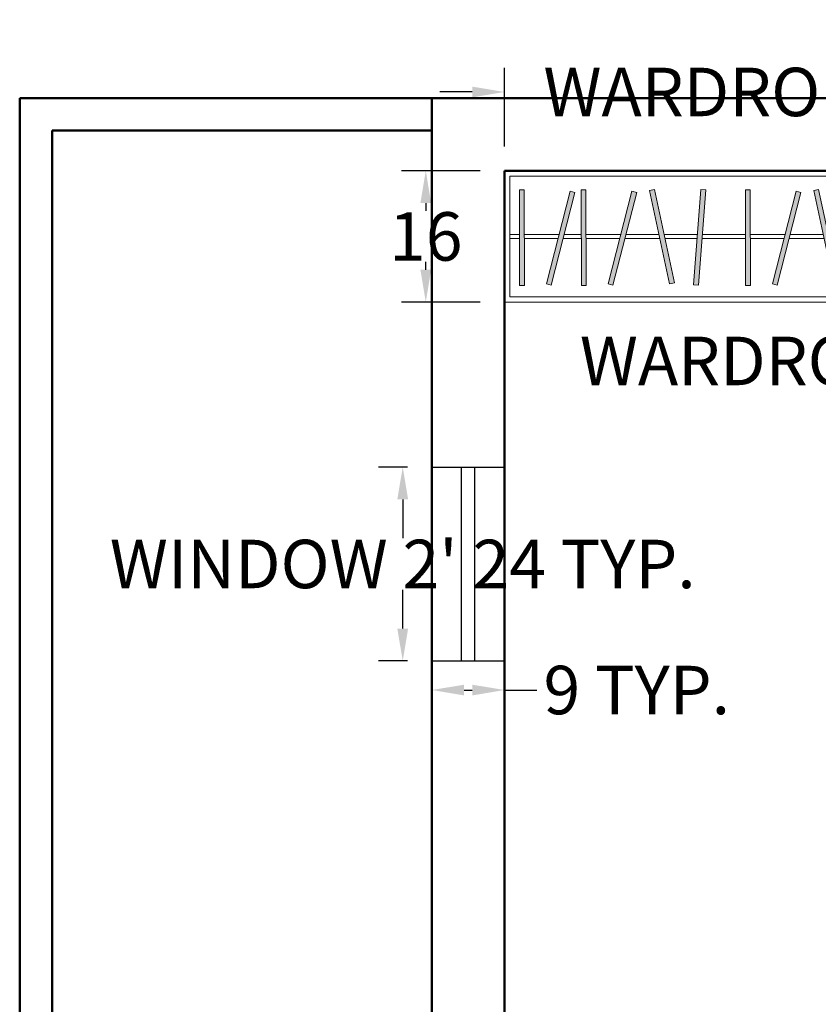
# Model space of a CAD drawing. Units: inches. Extents: x -466983 to 1020, y 324 to 318697.
# Tile 45 of 97: x 392 to 491, y 973 to 1095. Entities that reach past the tile are written whole.
import ezdxf

# ---------------------------------------------------------------- set-up
doc = ezdxf.new("R2010")
doc.units = ezdxf.units.IN
doc.header["$MEASUREMENT"] = 0
for name, color, linetype, lineweight in [('A-ANNO-DIMS', 2, 'Continuous', 18), ('A-ANNO-TEXT', 7, 'Continuous', 18), ('A-FLOR-PATT', 252, 'Continuous', 13), ('A-FURN', 8, 'Continuous', 18), ('A-GLAZ', 4, 'Continuous', 25), ('A-WALL', 7, 'Continuous', 50)]:
    doc.layers.add(name, color=color, linetype=linetype, lineweight=lineweight)
doc.styles.get("Standard").update_dxf_attribs({"font": 'arial.ttf'})
doc.dimstyles.get("Standard").update_dxf_attribs({"dimtxt": 6, "dimasz": 4, "dimexe": 3, "dimexo": 3, "dimgap": 0.09, "dimtad": 0, "dimtih": 1, "dimtoh": 1, "dimdec": 1, "dimzin": 0, "dimdsep": 46, "dimlunit": 3, "dimtxsty": 'Standard', "dimcen": 0.09, "dimadec": 0, "dimazin": 0, "dimtfac": 1, "dimtdec": 1, "dimtofl": 0, "dimtmove": 0, "dimatfit": 3, "dimfxl": 1, "dimtolj": 1, "dimtzin": 0, "dimarcsym": 0})

# ---------------------------------------------------------------- blocks, each defined once
blk = doc.blocks.new('Window 2 ft')
for p, q in [((1298.68, 816.59), (1322.68, 816.59)), ((1298.68, 807.59), (1298.68, 816.59)), ((1322.68, 816.59), (1322.68, 807.59)), ((1298.68, 812.89), (1322.68, 812.89)), ((1322.68, 811.29), (1298.68, 811.29)), ((1322.68, 807.59), (1298.68, 807.59))]:
    blk.add_line(p, q)
blk = doc.blocks.new('Wardrobe 1.1')
h = blk.add_hatch(color=256)
h.dxf.hatch_style = 1
h.paths.add_polyline_path([(3151.3, 1187.5), (3169.8, 1187.5), (3168.9, 1551.7), (3150.3, 1551.6)])
h = blk.add_hatch(color=256)
h.dxf.hatch_style = 1
h.paths.add_polyline_path([(3361.9, 1541.7), (3343.9, 1546.3), (3253, 1193.6), (3270.9, 1189)])
h = blk.add_hatch(color=256)
h.dxf.hatch_style = 1
h.paths.add_polyline_path([(3403.9, 1551.7), (3385.4, 1551.6), (3386.3, 1187.5), (3404.8, 1187.5)])
h = blk.add_hatch(color=256)
h.dxf.hatch_style = 1
h.paths.add_polyline_path([(3596.9, 1541.7), (3579, 1546.3), (3488, 1193.6), (3506, 1189)])
h = blk.add_hatch(color=256)
h.dxf.hatch_style = 1
h.paths.add_polyline_path([(3664.2, 1553.1), (3646.1, 1549.2), (3722.5, 1193.1), (3740.6, 1197)])
h = blk.add_hatch(color=256)
h.dxf.hatch_style = 1
h.paths.add_polyline_path([(3813.8, 1190.3), (3832.3, 1188.9), (3859.6, 1552.1), (3841.1, 1553.5)])
h = blk.add_hatch(color=256)
h.dxf.hatch_style = 1
h.paths.add_polyline_path([(4029.4, 1551.7), (4010.9, 1551.6), (4011.8, 1187.5), (4030.3, 1187.5)])
h = blk.add_hatch(color=256)
h.dxf.hatch_style = 1
h.paths.add_polyline_path([(4222.4, 1541.7), (4204.5, 1546.3), (4113.5, 1193.6), (4131.5, 1189)])
h = blk.add_hatch(color=256)
h.dxf.hatch_style = 1
h.paths.add_polyline_path([(4348, 1193.1), (4366.1, 1197), (4289.7, 1553.1), (4271.6, 1549.2)])
h = blk.add_hatch(color=256)
h.dxf.hatch_style = 1
h.paths.add_polyline_path([(4623.6, 1559.1), (4605.5, 1555.6), (4674.4, 1198), (4692.6, 1201.5)])
h = blk.add_hatch(color=256)
h.dxf.hatch_style = 1
h.paths.add_polyline_path([(4837.6, 1550.3), (4819.3, 1553.2), (4762, 1193.5), (4780.3, 1190.6)])
h = blk.add_hatch(color=256)
h.dxf.hatch_style = 1
h.paths.add_polyline_path([(4895.9, 1554.7), (4877.4, 1553.3), (4902.7, 1196.8), (4921.1, 1198.1)])
h = blk.add_hatch(color=256)
h.dxf.hatch_style = 1
h.paths.add_polyline_path([(4989.4, 1559.9), (4970.9, 1559.9), (4971.8, 1195.7), (4990.3, 1195.7)])
at = {"ltscale": 5}
for p, q in [((3093.8, 1124.1), (3093.8, 1624.1)), ((3093.8, 1624.1), (5093.8, 1624.1)), ((5093.8, 1624.1), (5093.8, 1124.1)), ((5093.8, 1124.1), (3093.8, 1124.1))]:
    blk.add_line(p, q, dxfattribs=at)
for p, q in [((3113.8, 1144.1), (3113.8, 1604.1)), ((3113.8, 1604.1), (5073.8, 1604.1)), ((5073.8, 1604.1), (5073.8, 1144.1)), ((3168.9, 1551.7), (3150.3, 1551.6)), ((3150.3, 1551.6), (3151.3, 1187.5)), ((3169.8, 1187.5), (3168.9, 1551.7)), ((3343.9, 1546.3), (3253, 1193.6)), ((3270.9, 1189), (3361.9, 1541.7)), ((3361.9, 1541.7), (3343.9, 1546.3)), ((3403.9, 1551.7), (3385.4, 1551.6)), ((3385.4, 1551.6), (3386.3, 1187.5)), ((3404.8, 1187.5), (3403.9, 1551.7)), ((3579, 1546.3), (3488, 1193.6)), ((3506, 1189), (3596.9, 1541.7)), ((3596.9, 1541.7), (3579, 1546.3)), ((3664.2, 1553.1), (3646.1, 1549.2)), ((3646.1, 1549.2), (3722.5, 1193.1)), ((3740.6, 1197), (3664.2, 1553.1)), ((3841.1, 1553.5), (3813.8, 1190.3)), ((3832.3, 1188.9), (3859.6, 1552.1)), ((3859.6, 1552.1), (3841.1, 1553.5)), ((4029.4, 1551.7), (4010.9, 1551.6)), ((4010.9, 1551.6), (4011.8, 1187.5)), ((4030.3, 1187.5), (4029.4, 1551.7)), ((4204.5, 1546.3), (4113.5, 1193.6)), ((4131.5, 1189), (4222.4, 1541.7)), ((4222.4, 1541.7), (4204.5, 1546.3)), ((4289.7, 1553.1), (4271.6, 1549.2)), ((4271.6, 1549.2), (4348, 1193.1)), ((4366.1, 1197), (4289.7, 1553.1)), ((4623.6, 1559.1), (4605.5, 1555.6)), ((4605.5, 1555.6), (4674.4, 1198)), ((4692.6, 1201.5), (4623.6, 1559.1)), ((4819.3, 1553.2), (4762, 1193.5)), ((4780.3, 1190.6), (4837.6, 1550.3)), ((4837.6, 1550.3), (4819.3, 1553.2)), ((4895.9, 1554.7), (4877.4, 1553.3)), ((4877.4, 1553.3), (4902.7, 1196.8)), ((4921.1, 1198.1), (4895.9, 1554.7)), ((4970.9, 1559.9), (4971.8, 1195.7)), ((4989.4, 1559.9), (4970.9, 1559.9)), ((4990.3, 1195.7), (4989.4, 1559.9)), ((3150.8, 1382.1), (3113.8, 1382.1)), ((3150.8, 1366.1), (3113.8, 1366.1)), ((3301.6, 1382.1), (3169.3, 1382.1)), ((3301.6, 1382.1), (3169.3, 1382.1)), ((3297.5, 1366.1), (3169.3, 1366.1)), ((3297.5, 1366.1), (3169.3, 1366.1)), ((3385.9, 1366.1), (3316.6, 1366.1)), ((3385.8, 1382.1), (3320.7, 1382.1)), ((3536.6, 1382.1), (3404.3, 1382.1)), ((3536.6, 1382.1), (3404.3, 1382.1)), ((3532.5, 1366.1), (3404.4, 1366.1)), ((3532.5, 1366.1), (3404.4, 1366.1)), ((3685.4, 1366.1), (3551.6, 1366.1)), ((3685.4, 1366.1), (3551.6, 1366.1)), ((3682, 1382.1), (3555.8, 1382.1)), ((3682, 1382.1), (3555.8, 1382.1)), ((3828.3, 1382.1), (3700.9, 1382.1)), ((3828.3, 1382.1), (3700.9, 1382.1)), ((3827, 1366.1), (3704.3, 1366.1)), ((3827, 1366.1), (3704.3, 1366.1)), ((4011.4, 1366.1), (3845.6, 1366.1)), ((4011.3, 1382.1), (3846.8, 1382.1)), ((4162.1, 1382.1), (4029.8, 1382.1)), ((4158, 1366.1), (4029.9, 1366.1)), ((4310.9, 1366.1), (4177.1, 1366.1)), ((4307.5, 1382.1), (4181.3, 1382.1)), ((4453.8, 1382.1), (4326.4, 1382.1)), ((4452.6, 1366.1), (4329.8, 1366.1)), ((4642, 1366.1), (4471.1, 1366.1)), ((4638.9, 1382.1), (4472.3, 1382.1)), ((4792.1, 1382.1), (4657.8, 1382.1)), ((4789.5, 1366.1), (4660.9, 1366.1)), ((4890.7, 1366.1), (4808.3, 1366.1)), ((4889.5, 1382.1), (4810.8, 1382.1)), ((4971.3, 1382.1), (4908.1, 1382.1)), ((4971.4, 1366.1), (4909.2, 1366.1)), ((5073.8, 1382.1), (4989.8, 1382.1)), ((5073.8, 1366.1), (4989.9, 1366.1)), ((4674.4, 1198), (4692.6, 1201.5)), ((3169.8, 1187.5), (3151.3, 1187.5)), ((3253, 1193.6), (3270.9, 1189)), ((3404.8, 1187.5), (3386.3, 1187.5)), ((3488, 1193.6), (3506, 1189)), ((3722.5, 1193.1), (3740.6, 1197)), ((3832.3, 1188.9), (3813.8, 1190.3)), ((4030.3, 1187.5), (4011.8, 1187.5)), ((4113.5, 1193.6), (4131.5, 1189)), ((4348, 1193.1), (4366.1, 1197)), ((4762, 1193.5), (4780.3, 1190.6)), ((4902.7, 1196.8), (4921.1, 1198.1)), ((4971.8, 1195.7), (4990.3, 1195.7)), ((5073.8, 1144.1), (3113.8, 1144.1))]:
    blk.add_line(p, q)
blk.add_lwpolyline([(4439.3, 1190.3), (4466.6, 1553.5), (4485.1, 1552.1), (4457.8, 1188.9), (4439.2, 1188.9)])
blk = doc.blocks.new('*D63')
at = {"layer": 'A-ANNO-DIMS', "color": 0, "lineweight": -2, "transparency": 16777216}
for p, q in [((439.81, 1039.27), (436.21, 1039.27)), ((439.21, 1035.27), (439.21, 1030.46)), ((439.21, 1019.27), (439.21, 1024.07)), ((439.81, 1015.27), (436.21, 1015.27))]:
    blk.add_line(p, q, dxfattribs=at)
at = {"layer": 'A-ANNO-DIMS', "color": 0, "transparency": 16777216}
for points in [[(438.54, 1035.27), (439.87, 1035.27), (439.21, 1039.27)], [(438.54, 1019.27), (439.87, 1019.27), (439.21, 1015.27)]]:
    blk.add_solid(points, dxfattribs=at)
at = {"layer": 'Defpoints', "color": 0, "transparency": 16777216}
for p in [(442.81, 1039.27), (439.21, 1015.27), (442.81, 1015.27)]:
    blk.add_point(p, dxfattribs=at)
at = {"layer": 'A-ANNO-DIMS', "color": 0, "transparency": 16777216, "insert": (439.21, 1027.27), "char_height": 6, "attachment_point": 5}
blk.add_mtext("\\A1;WINDOW 2' 24 TYP.", dxfattribs=at)
blk = doc.blocks.new('*D64')
at = {"layer": 'A-ANNO-DIMS', "color": 0, "lineweight": -2, "transparency": 16777216}
for p, q in [((442.81, 1012.27), (442.81, 1008.67)), ((446.81, 1011.67), (447.81, 1011.67)), ((451.81, 1012.27), (451.81, 1008.67)), ((451.81, 1011.67), (455.81, 1011.67))]:
    blk.add_line(p, q, dxfattribs=at)
at = {"layer": 'A-ANNO-DIMS', "color": 0, "transparency": 16777216}
for points in [[(446.81, 1012.33), (446.81, 1011), (442.81, 1011.67)], [(447.81, 1012.33), (447.81, 1011), (451.81, 1011.67)]]:
    blk.add_solid(points, dxfattribs=at)
at = {"layer": 'Defpoints', "color": 0, "transparency": 16777216}
for p in [(442.81, 1015.27), (451.81, 1015.27), (451.81, 1011.67)]:
    blk.add_point(p, dxfattribs=at)
at = {"layer": 'A-ANNO-DIMS', "color": 0, "transparency": 16777216, "insert": (468.17, 1011.67), "char_height": 6, "attachment_point": 5}
blk.add_mtext('\\A1;9 TYP.', dxfattribs=at)
blk = doc.blocks.new('*D83')
at = {"layer": 'A-ANNO-DIMS', "color": 0, "lineweight": -2, "transparency": 16777216}
for p, q in [((451.81, 1078.94), (451.81, 1088.69)), ((516.81, 1078.94), (516.81, 1088.69)), ((447.81, 1085.69), (443.81, 1085.69)), ((520.81, 1085.69), (524.81, 1085.69))]:
    blk.add_line(p, q, dxfattribs=at)
at = {"layer": 'A-ANNO-DIMS', "color": 0, "transparency": 16777216}
for points in [[(447.81, 1086.35), (447.81, 1085.02), (451.81, 1085.69)], [(520.81, 1086.35), (520.81, 1085.02), (516.81, 1085.69)]]:
    blk.add_solid(points, dxfattribs=at)
at = {"layer": 'Defpoints', "color": 0, "transparency": 16777216}
for p in [(516.81, 1085.69), (451.81, 1075.94), (516.81, 1075.94)]:
    blk.add_point(p, dxfattribs=at)
at = {"layer": 'A-ANNO-DIMS', "color": 0, "transparency": 16777216, "insert": (484.31, 1085.69), "char_height": 6, "attachment_point": 5}
blk.add_mtext('\\A1;WARDROBE 65', dxfattribs=at)
blk = doc.blocks.new('*D84')
at = {"layer": 'A-ANNO-DIMS', "color": 0, "lineweight": -2, "transparency": 16777216}
for p, q in [((448.81, 1075.94), (439.06, 1075.94)), ((442.06, 1071.94), (442.06, 1070.97)), ((442.06, 1063.69), (442.06, 1064.66)), ((448.81, 1059.69), (439.06, 1059.69))]:
    blk.add_line(p, q, dxfattribs=at)
at = {"layer": 'A-ANNO-DIMS', "color": 0, "transparency": 16777216}
for points in [[(441.39, 1071.94), (442.72, 1071.94), (442.06, 1075.94)], [(441.39, 1063.69), (442.72, 1063.69), (442.06, 1059.69)]]:
    blk.add_solid(points, dxfattribs=at)
at = {"layer": 'Defpoints', "color": 0, "transparency": 16777216}
for p in [(442.06, 1075.94), (451.81, 1075.94), (451.81, 1059.69)]:
    blk.add_point(p, dxfattribs=at)
at = {"layer": 'A-ANNO-DIMS', "color": 0, "transparency": 16777216, "insert": (442.06, 1067.81), "char_height": 6, "attachment_point": 5}
blk.add_mtext('\\A1;16', dxfattribs=at)

msp = doc.modelspace()

# ---------------------------------------------------------------- hatches: boundary and pattern name
at = {"layer": 'A-FLOR-PATT', "transparency": 33554572}
h = msp.add_hatch(dxfattribs=at)
h.set_pattern_fill('ANSI37', color=256, scale=30)
h.set_pattern_definition([(45, (-1212.4137, -290.035), (-2.6516504, 2.6516504), []), (135, (-1212.4137, -290.035), (-2.6516504, -2.6516504), [])])
h.paths.add_polyline_path([(901.81, 1075.94), (900.61, 1075.94), (900.61, 1065.39), (899.39, 1065.39), (898.09, 1065.39), (892.84, 1058.71, -0.258377), (892.19, 1058.35), (879.98, 1058.35, -0.20177), (879.44, 1058.58), (874.08, 1065.39), (872.78, 1065.39), (871.56, 1065.39), (871.56, 1075.94), (813.81, 1075.94), (813.81, 1044.79), (832.39, 1044.79, -0.394795), (848.66, 1028.54), (848.66, 1009.94), (901.81, 1009.94), (901.81, 1015.94), (901.31, 1015.94), (871.31, 1015.94), (871.31, 1017.25), (871.33, 1017.25, -0.401453), (901.31, 1045.94), (901.81, 1045.94)])
edge = h.paths.add_edge_path(flags=16)
edge.add_line((847.77, 1068.95), (847.77, 1073.71))
edge.add_arc((849.23, 1073.71), 1.45, 90, 180, ccw=False)
edge.add_line((849.23, 1075.16), (864.49, 1075.16))
edge.add_arc((864.49, 1073.71), 1.45, 0, 90, ccw=False)
edge.add_line((865.95, 1073.71), (865.95, 1069))
edge.add_arc((832.64, 1068.98), 33.3, -20.6123, 0.0472, ccw=False)
edge.add_ellipse((856.86, 1058.48), major_axis=(0, 10.21), ratio=0.685919, start_angle=100.0088, end_angle=259.9912, ccw=False)
edge.add_arc((881.07, 1068.98), 33.3, 180.0472, 200.6123, ccw=False)
h.paths.add_polyline_path([(853.15, 1066.48), (853.15, 1066.45), (853.15, 1066.45, 0.433107), (852.92, 1066.68), (852.92, 1066.45), (853.15, 1066.45), (853.15, 1066.48), (853.09, 1066.61, 0.697939), (852.7, 1066.45), (852.7, 1066.45), (852.7, 1066.48), (852.92, 1067), (852.92, 1066.68, -0.396254)], flags=0)
h.paths.add_polyline_path([(861.02, 1066.48), (861.02, 1066.45), (861.02, 1066.45, 0.416404), (860.8, 1066.68), (860.8, 1066.45), (861.02, 1066.45), (861.02, 1066.48), (860.97, 1066.61, 0.713344), (860.57, 1066.45), (860.57, 1066.45), (860.57, 1066.48), (860.8, 1067), (860.8, 1066.68, -0.379973)], flags=0)
edge = h.paths.add_edge_path(flags=0)
edge.add_spline(control_points=[(861.13, 1065.79), (861.47, 1065.25), (861.61, 1065.02), (861.98, 1064.37), (862.19, 1063.94), (862.56, 1063.04), (862.72, 1062.56), (862.99, 1061.58), (863.09, 1061.07), (863.25, 1060.03), (863.29, 1059.5), (863.33, 1058.44), (863.32, 1057.91), (863.24, 1056.85), (863.17, 1056.33), (862.97, 1055.31), (862.84, 1054.81), (862.54, 1053.85), (862.36, 1053.39), (861.95, 1052.52), (861.73, 1052.12), (861.23, 1051.36), (860.97, 1051.02), (860.4, 1050.39), (860.11, 1050.12), (859.49, 1049.65), (859.18, 1049.45), (858.53, 1049.13), (858.2, 1049.01), (857.53, 1048.85), (857.2, 1048.81), (856.52, 1048.81), (856.19, 1048.85), (855.52, 1049.01), (855.19, 1049.13), (854.54, 1049.45), (854.23, 1049.64), (853.61, 1050.12), (853.32, 1050.39), (852.75, 1051.01), (852.49, 1051.36), (852, 1052.11), (851.77, 1052.52), (851.36, 1053.39), (851.18, 1053.85), (850.88, 1054.81), (850.75, 1055.31), (850.55, 1056.33), (850.48, 1056.85), (850.4, 1057.9), (850.39, 1058.44), (850.43, 1059.5), (850.47, 1060.03), (850.63, 1061.07), (850.73, 1061.58), (851, 1062.56), (851.16, 1063.04), (851.53, 1063.94), (851.73, 1064.37), (852.11, 1065.02), (852.25, 1065.25), (852.61, 1065.73)], knot_values=[3.915332, 3.915332, 3.915332, 3.915332, 4.013468, 4.013468, 4.175532, 4.175532, 4.337596, 4.337596, 4.49966, 4.49966, 4.661724, 4.661724, 4.823788, 4.823788, 4.985852, 4.985852, 5.147916, 5.147916, 5.30998, 5.30998, 5.472044, 5.472044, 5.634109, 5.634109, 5.796173, 5.796173, 5.958237, 5.958237, 6.120301, 6.120301, 6.282365, 6.282365, 6.444429, 6.444429, 6.606493, 6.606493, 6.768557, 6.768557, 6.930621, 6.930621, 7.092685, 7.092685, 7.254749, 7.254749, 7.416813, 7.416813, 7.578878, 7.578878, 7.740942, 7.740942, 7.903006, 7.903006, 8.06507, 8.06507, 8.227134, 8.227134, 8.389198, 8.389198, 8.551262, 8.551262, 8.65037, 8.65037, 8.65037, 8.65037], degree=3, periodic=0)
edge.add_line((852.64, 1065.79), (861.13, 1065.79))
edge = h.paths.add_edge_path(flags=0)
edge.add_ellipse((856.85, 1057.74), major_axis=(0, 7.79), ratio=0.687861, start_angle=0, end_angle=360)
h.paths.add_polyline_path([(848.86, 1069.39), (848.86, 1073.96, -0.414214), (849.95, 1075.05), (863.77, 1075.05, -0.414214), (864.86, 1073.96), (864.86, 1069.39, -0.388936), (864.52, 1069.03, -0.043561), (849.2, 1069.03, -0.388936)], flags=0)
h.paths.add_polyline_path([(853.1, 1068.11, -1), (852.68, 1068.11, -1)], flags=0)
edge = h.paths.add_edge_path(flags=0)
edge.add_ellipse((856.86, 1057.34), major_axis=(0, 2.21), ratio=0.657164, start_angle=0, end_angle=360)
h.paths.add_polyline_path([(861.04, 1068.11, -1), (860.62, 1068.11, -1)], flags=0)
edge = h.paths.add_edge_path()
edge.add_line((573.95, 1057.34), (573.95, 1075.94))
edge.add_line((573.95, 1075.94), (558.73, 1075.94))
edge.add_line((558.73, 1075.94), (558.73, 1065.39))
edge.add_line((558.73, 1065.39), (557.51, 1065.39))
edge.add_line((557.51, 1065.39), (556.21, 1065.39))
edge.add_line((556.21, 1065.39), (550.95, 1058.71))
edge.add_arc((550.3, 1059.12), 0.765, 270, 327.9483, ccw=False)
edge.add_line((550.3, 1058.35), (538.1, 1058.35))
edge.add_arc((538.1, 1059.12), 0.765, 224.3704, 270, ccw=False)
edge.add_line((537.55, 1058.58), (532.2, 1065.39))
edge.add_line((532.2, 1065.39), (530.9, 1065.39))
edge.add_line((530.9, 1065.39), (529.67, 1065.39))
edge.add_line((529.67, 1065.39), (529.67, 1075.94))
edge.add_line((529.67, 1075.94), (520.81, 1075.94))
edge.add_line((520.81, 1075.94), (520.81, 1045.94))
edge.add_line((520.81, 1045.94), (521.31, 1045.94))
edge.add_arc((521.31, 1015.94), 30, 2.5075, 90, ccw=False)
edge.add_line((551.28, 1017.25), (551.31, 1017.25))
edge.add_line((551.31, 1017.25), (551.31, 1015.94))
edge.add_line((551.31, 1015.94), (520.81, 1015.94))
edge.add_line((520.81, 1015.94), (520.81, 1009.94))
edge.add_line((520.81, 1009.94), (559.19, 1010.4))
edge.add_arc((559.19, 1011.86), 1.45, 180, 270, ccw=False)
edge.add_line((557.74, 1011.86), (557.74, 1016.56))
edge.add_arc((591.04, 1016.59), 33.3, 159.3877, 180.0472, ccw=False)
edge.add_ellipse((566.82, 1027.08), major_axis=(0, 10.21), ratio=0.685919, start_angle=280.0088, end_angle=439.9912, ccw=False)
edge.add_arc((542.61, 1016.59), 33.3, 0.0472, 20.6123, ccw=False)
edge.add_line((575.91, 1016.62), (575.91, 1011.86))
edge.add_arc((574.46, 1011.86), 1.45, -90, 0, ccw=False)
edge.add_line((574.46, 1010.4), (608.81, 1009.94))
edge.add_line((608.81, 1009.94), (608.81, 1041.09))
edge.add_line((608.81, 1041.09), (590.22, 1041.09))
edge.add_arc((590.78, 1057.91), 16.83, 181.9277, 268.1032, ccw=False)
edge = h.paths.add_edge_path()
edge.add_ellipse((494.24, 583.62), major_axis=(0, 10.21), ratio=0.685919, start_angle=280.0088, end_angle=439.9912, ccw=False)
edge.add_arc((470.03, 573.12), 33.3, 0.0472, 20.6123, ccw=False)
edge.add_line((503.33, 573.15), (503.33, 568.39))
edge.add_arc((501.88, 568.39), 1.45, -90, 0, ccw=False)
edge.add_line((501.88, 566.94), (539.81, 566.94))
edge.add_line((539.81, 566.94), (539.81, 572.94))
edge.add_line((539.81, 572.94), (539.31, 572.94))
edge.add_line((539.31, 572.94), (509.31, 572.94))
edge.add_line((509.31, 572.94), (509.31, 574.25))
edge.add_line((509.31, 574.25), (509.33, 574.25))
edge.add_arc((539.31, 572.94), 30, 90, 177.4925, ccw=False)
edge.add_line((539.31, 602.94), (539.81, 602.94))
edge.add_line((539.81, 602.94), (539.81, 626.94))
edge.add_line((539.81, 626.94), (531.77, 626.94))
edge.add_line((531.77, 626.94), (531.77, 616.39))
edge.add_line((531.77, 616.39), (530.55, 616.39))
edge.add_line((530.55, 616.39), (529.25, 616.39))
edge.add_line((529.25, 616.39), (523.71, 609.35))
edge.add_line((523.71, 609.35), (510.78, 609.35))
edge.add_line((510.78, 609.35), (505.24, 616.39))
edge.add_line((505.24, 616.39), (503.94, 616.39))
edge.add_line((503.94, 616.39), (502.72, 616.39))
edge.add_line((502.72, 616.39), (502.72, 626.94))
edge.add_line((502.72, 626.94), (481.7, 626.94))
edge.add_line((481.7, 626.94), (481.7, 611))
edge.add_arc((467.27, 611.47), 14.44, 271.9277, 358.1032, ccw=False)
edge.add_line((467.76, 597.05), (451.81, 597.05))
edge.add_line((451.81, 597.05), (451.81, 584.4))
edge.add_line((451.81, 584.4), (451.81, 566.94))
edge.add_line((451.81, 566.94), (486.61, 566.94))
edge.add_arc((486.61, 568.39), 1.45, 180, 270, ccw=False)
edge.add_line((485.16, 568.39), (485.16, 573.1))
edge.add_arc((518.46, 573.12), 33.3, 159.3877, 180.0472, ccw=False)
h.paths.add_polyline_path([(836.26, 1020.73), (879.89, 1020.73), (879.89, 1039.39), (836.26, 1039.39)], flags=25)
h.paths.add_polyline_path([(549.99, 1036.75), (593.61, 1036.75), (593.61, 1055.41), (549.99, 1055.41)], flags=24)
h.paths.add_polyline_path([(475.12, 595.6), (518.75, 595.6), (518.75, 614.25), (475.12, 614.25)], flags=24)

# ---------------------------------------------------------------- linework, layer by layer
at = {"layer": 'A-WALL'}
for p, q in [((391.81, 1084.94), (991.81, 1084.94)), ((391.81, 364.94), (391.81, 1084.94)), ((442.81, 415.94), (442.81, 1084.94)), ((395.81, 1080.94), (442.81, 1080.94)), ((395.81, 368.94), (395.81, 1080.94)), ((451.81, 1075.94), (516.81, 1075.94)), ((451.81, 828.94), (451.81, 1075.94))]:
    msp.add_line(p, q, dxfattribs=at)

# ---------------------------------------------------------------- block references
at = {"layer": 'A-FURN', "xscale": 0.0325, "yscale": 0.0325, "zscale": 0.0325}
msp.add_blockref('Wardrobe 1.1', (351.26, 1023.15), dxfattribs=at)
at = {"layer": 'A-GLAZ', "rotation": 270}
msp.add_blockref('Window 2 ft', (-364.79, 2337.94), dxfattribs=at)

# ---------------------------------------------------------------- texts
at = {"layer": 'A-ANNO-TEXT', "insert": (368.58, 1055.4), "char_height": 6, "attachment_point": 1}
msp.add_mtext_dynamic_manual_height_columns('\\pxqc;WARDROBE', width=229.5583, gutter_width=1, heights=[0], dxfattribs=at)

# ---------------------------------------------------------------- dimensions: what is measured, and where the dimension line sits
at = {"layer": 'A-ANNO-DIMS'}
for base, p1, p2, text, picture, middle in [((516.81, 1085.69), (451.81, 1075.94), (516.81, 1075.94), 'WARDROBE <>', '*D83', (484.31, 1085.69)), ((451.81, 1011.67), (442.81, 1015.27), (451.81, 1015.27), '<> TYP.', '*D64', (468.17, 1011.67))]:
    dim = msp.add_linear_dim(base=base, p1=p1, p2=p2, text=text, dimstyle='Standard', override={"dimdec": 0, "dimlfac": 1, "dimrnd": 0, "dimzin": 0, "dimdsep": 46, "dimlunit": 2}, dxfattribs=at)
    dim.commit()
    dim.dimension.update_dxf_attribs({"geometry": picture, "text_midpoint": middle})
dim = msp.add_linear_dim(base=(442.06, 1075.94), p1=(451.81, 1059.69), p2=(451.81, 1075.94), angle=90, dimstyle='Standard', override={"dimdec": 0, "dimlfac": 1, "dimrnd": 0, "dimzin": 0, "dimdsep": 46, "dimlunit": 2}, dxfattribs=at)
dim.commit()
dim.dimension.update_dxf_attribs({"geometry": '*D84', "text_midpoint": (442.06, 1067.81)})
dim = msp.add_linear_dim(base=(439.21, 1015.27), p1=(442.81, 1039.27), p2=(442.81, 1015.27), angle=270, text="WINDOW 2' <> TYP.", dimstyle='Standard', override={"dimdec": 0, "dimlfac": 1, "dimrnd": 0, "dimzin": 0, "dimdsep": 46, "dimlunit": 2}, dxfattribs=at)
dim.commit()
dim.dimension.update_dxf_attribs({"geometry": '*D63', "text_midpoint": (439.21, 1027.27)})

doc.saveas('drawing.dxf')
